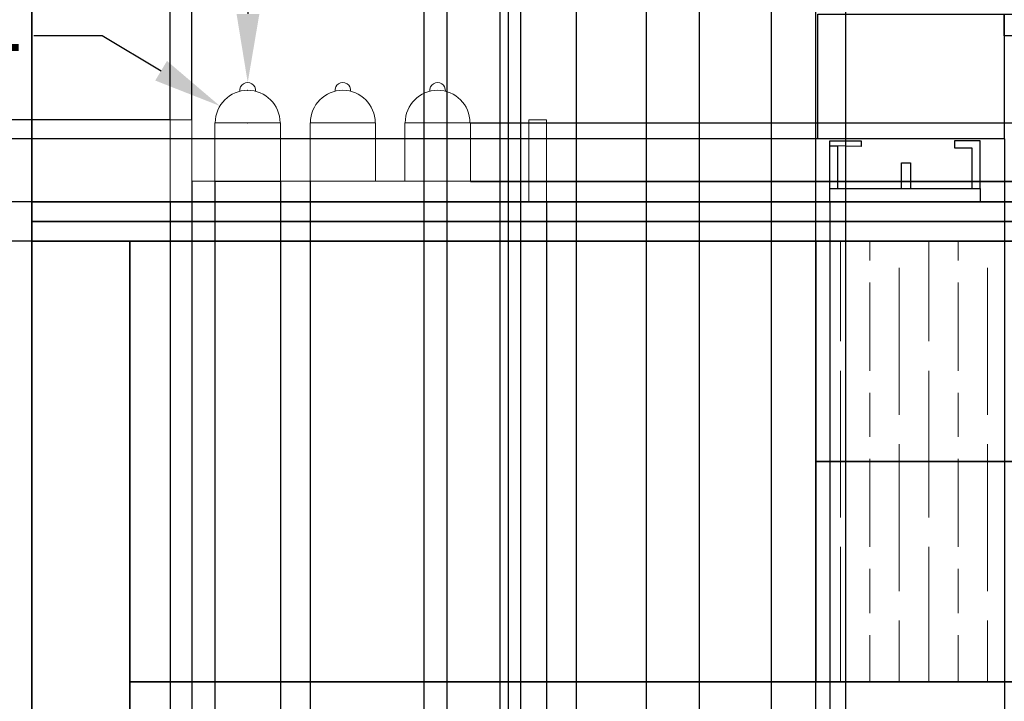
# Model space of a CAD drawing. Units: inches. Extents: x 600 to 5582, y -464 to 3142.
# Tile 3 of 9: x 1772 to 2777, y 532 to 1229. Entities that reach past the tile are written whole.
import ezdxf

# ---------------------------------------------------------------- set-up
doc = ezdxf.new("R2010")
doc.units = ezdxf.units.IN
doc.header["$MEASUREMENT"] = 0
for name, color, linetype, lineweight in [('A-ANNO-DIMS', 2, 'Continuous', 18), ('A-ELEV', 7, 'Continuous', 35), ('A-ELEV-PATT', 252, 'Continuous', 13), ('A-EQPM', 4, 'Continuous', 25), ('A-FURN', 8, 'Continuous', 18)]:
    doc.layers.add(name, color=color, linetype=linetype, lineweight=lineweight)
doc.styles.get("Standard").update_dxf_attribs({"font": 'arial.ttf'})
doc.dimstyles.get("Standard").update_dxf_attribs({"dimtxt": 70, "dimasz": 70, "dimexe": 0.18, "dimexo": 0.0625, "dimgap": 0.09, "dimtad": 0, "dimtih": 1, "dimtoh": 1, "dimdec": 0, "dimzin": 0, "dimdsep": 46, "dimtxsty": 'Standard', "dimcen": 0.09, "dimadec": 0, "dimazin": 0, "dimtfac": 1, "dimtdec": 0, "dimtofl": 0, "dimtmove": 0, "dimatfit": 3, "dimfxl": 1, "dimtolj": 1, "dimtzin": 0, "dimarcsym": 0})

# ---------------------------------------------------------------- blocks, each defined once
blk = doc.blocks.new('HOB-BURNER')
for p, q in [((0, 13.8), (0, 62.4)), ((0, 62.4), (31.8, 62.4)), ((31.8, 62.4), (31.8, 56.6)), ((153.5, 62.4), (127.3, 62.4)), ((127.3, 62.4), (127.3, 55.3)), ((153.5, 13.8), (153.5, 62.4)), ((31.8, 56.6), (0, 57.4)), ((0, 57.4), (7.8, 57.2)), ((7.8, 57.2), (7.8, 13.8)), ((127.3, 55.3), (144.9, 55.3)), ((144.9, 55.3), (144.9, 13.8)), ((73.1, 13.8), (73.1, 39.8)), ((73.1, 39.8), (82.4, 39.8)), ((82.4, 39.8), (82.4, 13.8)), ((7.8, 13.8), (73.1, 13.8)), ((82.4, 13.8), (153.5, 13.8))]:
    blk.add_line(p, q)
blk.add_lwpolyline([(0, 13.8), (153.5, 13.8), (153.5, 0), (0, 0)], close=True)
blk = doc.blocks.new('*D25')
at = {"layer": 'A-ANNO-DIMS', "color": 0, "lineweight": -2, "transparency": 16777216}
for p, q in [((2584.7, 1680.8), (2584.7, -233.3)), ((2615, 1655.8), (2615, -233.3)), ((2514.7, -233.1), (2444.7, -233.1)), ((2685, -233.1), (2755, -233.1))]:
    blk.add_line(p, q, dxfattribs=at)
at = {"layer": 'A-ANNO-DIMS', "color": 0, "transparency": 16777216}
for points in [[(2514.7, -221.4), (2514.7, -244.7), (2584.7, -233.1)], [(2685, -221.4), (2685, -244.7), (2615, -233.1)]]:
    blk.add_solid(points, dxfattribs=at)
at = {"layer": 'Defpoints', "color": 0, "transparency": 16777216}
for p in [(2584.7, 1680.8), (2615, 1655.8), (2615, -233.1)]:
    blk.add_point(p, dxfattribs=at)
at = {"layer": 'A-ANNO-DIMS', "color": 0, "transparency": 16777216, "insert": (2873.3, -233.1), "char_height": 70, "attachment_point": 5}
blk.add_mtext('\\A1;30.28', dxfattribs=at)
blk = doc.blocks.new('*D57')
at = {"layer": 'A-ANNO-DIMS', "color": 0, "lineweight": -2, "transparency": 16777216}
for p, q in [((5220.2, 622.4), (5220.2, 692.4)), ((5220.2, 692.4), (5290.2, 692.4)), ((1884.8, 552.4), (5220.4, 552.4)), ((1884.8, 512.4), (5220.4, 512.4)), ((5220.2, 442.4), (5220.2, 372.4))]:
    blk.add_line(p, q, dxfattribs=at)
at = {"layer": 'A-ANNO-DIMS', "color": 0, "transparency": 16777216}
for points in [[(5208.6, 622.4), (5231.9, 622.4), (5220.2, 552.4)], [(5208.6, 442.4), (5231.9, 442.4), (5220.2, 512.4)]]:
    blk.add_solid(points, dxfattribs=at)
at = {"layer": 'Defpoints', "color": 0, "transparency": 16777216}
for p in [(1884.7, 552.4), (5220.2, 552.4), (1884.7, 512.4)]:
    blk.add_point(p, dxfattribs=at)
at = {"layer": 'A-ANNO-DIMS', "color": 0, "transparency": 16777216, "insert": (5341.8, 692.4), "char_height": 70, "attachment_point": 5}
blk.add_mtext('\\A1;40', dxfattribs=at)
blk = doc.blocks.new('*D65')
at = {"layer": 'A-ANNO-DIMS', "color": 0, "lineweight": -2, "transparency": 16777216}
for p, q in [((1784.7, 2352.4), (1784.7, -233.3)), ((2184.7, 2352.4), (2184.7, -233.3)), ((1714.7, -233.1), (1644.7, -233.1)), ((2254.7, -233.1), (2324.7, -233.1))]:
    blk.add_line(p, q, dxfattribs=at)
at = {"layer": 'A-ANNO-DIMS', "color": 0, "transparency": 16777216}
for points in [[(1714.7, -221.4), (1714.7, -244.7), (1784.7, -233.1)], [(2254.7, -221.4), (2254.7, -244.7), (2184.7, -233.1)]]:
    blk.add_solid(points, dxfattribs=at)
at = {"layer": 'Defpoints', "color": 0, "transparency": 16777216}
for p in [(1784.7, 2352.4), (2184.7, 2352.4), (2184.7, -233.1)]:
    blk.add_point(p, dxfattribs=at)
at = {"layer": 'A-ANNO-DIMS', "color": 0, "transparency": 16777216, "insert": (1984.7, -233.1), "char_height": 70, "attachment_point": 5}
blk.add_mtext('\\A1;400.00', dxfattribs=at)
blk = doc.blocks.new('*D68')
at = {"layer": 'A-ANNO-DIMS', "color": 0, "lineweight": -2, "transparency": 16777216}
for p, q in [((2777.3, 1106.8), (2777.3, -233.3)), ((2584.7, 1002.4), (2584.7, -233.3)), ((2654.7, -233.1), (2707.3, -233.1)), ((2777.3, -233.1), (2847.3, -233.1))]:
    blk.add_line(p, q, dxfattribs=at)
at = {"layer": 'A-ANNO-DIMS', "color": 0, "transparency": 16777216}
for points in [[(2654.7, -221.4), (2654.7, -244.7), (2584.7, -233.1)], [(2707.3, -221.4), (2707.3, -244.7), (2777.3, -233.1)]]:
    blk.add_solid(points, dxfattribs=at)
at = {"layer": 'Defpoints', "color": 0, "transparency": 16777216}
for p in [(2777.3, 1106.8), (2584.7, 1002.4), (2777.3, -233.1)]:
    blk.add_point(p, dxfattribs=at)
at = {"layer": 'A-ANNO-DIMS', "color": 0, "transparency": 16777216, "insert": (2982.6, -233.1), "char_height": 70, "attachment_point": 5}
blk.add_mtext('\\A1;192.51', dxfattribs=at)
blk = doc.blocks.new('*D70')
at = {"layer": 'A-ANNO-DIMS', "color": 0, "lineweight": -2, "transparency": 16777216}
for p, q in [((1149.2, 1176.8), (1149.2, 1246.8)), ((1149.2, 1246.8), (1219.2, 1246.8)), ((2586.9, 1106.8), (1149.1, 1106.8)), ((2599.2, 1042.4), (1149.1, 1042.4)), ((1149.2, 972.4), (1149.2, 902.4))]:
    blk.add_line(p, q, dxfattribs=at)
at = {"layer": 'A-ANNO-DIMS', "color": 0, "transparency": 16777216}
for points in [[(1137.6, 1176.8), (1160.9, 1176.8), (1149.2, 1106.8)], [(1137.6, 972.4), (1160.9, 972.4), (1149.2, 1042.4)]]:
    blk.add_solid(points, dxfattribs=at)
at = {"layer": 'Defpoints', "color": 0, "transparency": 16777216}
for p in [(1149.2, 1106.8), (2586.9, 1106.8), (2599.2, 1042.4)]:
    blk.add_point(p, dxfattribs=at)
at = {"layer": 'A-ANNO-DIMS', "color": 0, "transparency": 16777216, "insert": (1337.3, 1246.8), "char_height": 70, "attachment_point": 5}
blk.add_mtext('\\A1;64.42', dxfattribs=at)
blk = doc.blocks.new('*D73')
at = {"layer": 'A-ANNO-DIMS', "color": 0, "lineweight": -2, "transparency": 16777216}
for p, q in [((2599.2, 1042.4), (2599.2, -233.3)), ((2584.7, 1002.4), (2584.7, -233.3)), ((2514.7, -233.1), (2444.7, -233.1)), ((2669.2, -233.1), (2739.2, -233.1))]:
    blk.add_line(p, q, dxfattribs=at)
at = {"layer": 'A-ANNO-DIMS', "color": 0, "transparency": 16777216}
for points in [[(2514.7, -221.4), (2514.7, -244.7), (2584.7, -233.1)], [(2669.2, -221.4), (2669.2, -244.7), (2599.2, -233.1)]]:
    blk.add_solid(points, dxfattribs=at)
at = {"layer": 'Defpoints', "color": 0, "transparency": 16777216}
for p in [(2599.2, 1042.4), (2584.7, 1002.4), (2599.2, -233.1)]:
    blk.add_point(p, dxfattribs=at)
at = {"layer": 'A-ANNO-DIMS', "color": 0, "transparency": 16777216, "insert": (2854, -233.1), "char_height": 70, "attachment_point": 5}
blk.add_mtext('\\A1;14.50', dxfattribs=at)
blk = doc.blocks.new('*D74')
at = {"layer": 'A-ANNO-DIMS', "color": 0, "lineweight": -2, "transparency": 16777216}
for p, q in [((2599.2, 1042.4), (2599.2, -233.3)), ((2884.4, 1042.4), (2884.4, -233.3)), ((2669.2, -233.1), (2814.4, -233.1)), ((2884.4, -233.1), (2954.4, -233.1))]:
    blk.add_line(p, q, dxfattribs=at)
at = {"layer": 'A-ANNO-DIMS', "color": 0, "transparency": 16777216}
for points in [[(2669.2, -221.4), (2669.2, -244.7), (2599.2, -233.1)], [(2814.4, -221.4), (2814.4, -244.7), (2884.4, -233.1)]]:
    blk.add_solid(points, dxfattribs=at)
at = {"layer": 'Defpoints', "color": 0, "transparency": 16777216}
for p in [(2599.2, 1042.4), (2884.4, 1042.4), (2884.4, -233.1)]:
    blk.add_point(p, dxfattribs=at)
at = {"layer": 'A-ANNO-DIMS', "color": 0, "transparency": 16777216, "insert": (3100, -233.1), "char_height": 70, "attachment_point": 5}
blk.add_mtext('\\A1;285.12', dxfattribs=at)
blk = doc.blocks.new('*D75')
at = {"layer": 'A-ANNO-DIMS', "color": 0, "lineweight": -2, "transparency": 16777216}
for p, q in [((2884.4, 1042.4), (2884.4, -233.3)), ((3196.2, 1042.4), (3196.2, -233.3)), ((2814.4, -233.1), (2744.4, -233.1)), ((3266.2, -233.1), (3336.2, -233.1))]:
    blk.add_line(p, q, dxfattribs=at)
at = {"layer": 'A-ANNO-DIMS', "color": 0, "transparency": 16777216}
for points in [[(2814.4, -221.4), (2814.4, -244.7), (2884.4, -233.1)], [(3266.2, -221.4), (3266.2, -244.7), (3196.2, -233.1)]]:
    blk.add_solid(points, dxfattribs=at)
at = {"layer": 'Defpoints', "color": 0, "transparency": 16777216}
for p in [(2884.4, 1042.4), (3196.2, 1042.4), (3196.2, -233.1)]:
    blk.add_point(p, dxfattribs=at)
at = {"layer": 'A-ANNO-DIMS', "color": 0, "transparency": 16777216, "insert": (3040.3, -233.1), "char_height": 70, "attachment_point": 5}
blk.add_mtext('\\A1;311.87', dxfattribs=at)
blk = doc.blocks.new('*D76')
at = {"layer": 'A-ANNO-DIMS', "color": 0, "lineweight": -2, "transparency": 16777216}
for p, q in [((1149.2, 1112.4), (1149.2, 1182.4)), ((1149.2, 1182.4), (1219.2, 1182.4)), ((1784.7, 1042.4), (1149.1, 1042.4)), ((1784.7, 1002.4), (1149.1, 1002.4)), ((1149.2, 932.4), (1149.2, 862.4))]:
    blk.add_line(p, q, dxfattribs=at)
at = {"layer": 'A-ANNO-DIMS', "color": 0, "transparency": 16777216}
for points in [[(1137.6, 1112.4), (1160.9, 1112.4), (1149.2, 1042.4)], [(1137.6, 932.4), (1160.9, 932.4), (1149.2, 1002.4)]]:
    blk.add_solid(points, dxfattribs=at)
at = {"layer": 'Defpoints', "color": 0, "transparency": 16777216}
for p in [(1149.2, 1042.4), (1784.7, 1042.4), (1784.7, 1002.4)]:
    blk.add_point(p, dxfattribs=at)
at = {"layer": 'A-ANNO-DIMS', "color": 0, "transparency": 16777216, "insert": (1338.7, 1182.4), "char_height": 70, "attachment_point": 5}
blk.add_mtext('\\A1;40.00', dxfattribs=at)
blk = doc.blocks.new('*D77')
at = {"layer": 'A-ANNO-DIMS', "color": 0, "lineweight": -2, "transparency": 16777216}
for p, q in [((1784.7, 1042.4), (1784.7, -233.3)), ((1925.7, 1042.4), (1925.7, -233.3)), ((1854.7, -233.1), (1855.7, -233.1)), ((1925.7, -233.1), (1995.7, -233.1))]:
    blk.add_line(p, q, dxfattribs=at)
at = {"layer": 'A-ANNO-DIMS', "color": 0, "transparency": 16777216}
for points in [[(1854.7, -221.4), (1854.7, -244.7), (1784.7, -233.1)], [(1855.7, -221.4), (1855.7, -244.7), (1925.7, -233.1)]]:
    blk.add_solid(points, dxfattribs=at)
at = {"layer": 'Defpoints', "color": 0, "transparency": 16777216}
for p in [(1784.7, 1042.4), (1925.7, 1042.4), (1925.7, -233.1)]:
    blk.add_point(p, dxfattribs=at)
at = {"layer": 'A-ANNO-DIMS', "color": 0, "transparency": 16777216, "insert": (2138.1, -233.1), "char_height": 70, "attachment_point": 5}
blk.add_mtext('\\A1;140.95', dxfattribs=at)
blk = doc.blocks.new('*D78')
at = {"layer": 'A-ANNO-DIMS', "color": 0, "lineweight": -2, "transparency": 16777216}
for p, q in [((1925.7, 1042.4), (1925.7, -233.3)), ((2310, 1042.4), (2310, -233.3)), ((1855.7, -233.1), (1785.7, -233.1)), ((2380, -233.1), (2450, -233.1))]:
    blk.add_line(p, q, dxfattribs=at)
at = {"layer": 'A-ANNO-DIMS', "color": 0, "transparency": 16777216}
for points in [[(1855.7, -221.4), (1855.7, -244.7), (1925.7, -233.1)], [(2380, -221.4), (2380, -244.7), (2310, -233.1)]]:
    blk.add_solid(points, dxfattribs=at)
at = {"layer": 'Defpoints', "color": 0, "transparency": 16777216}
for p in [(1925.7, 1042.4), (2310, 1042.4), (2310, -233.1)]:
    blk.add_point(p, dxfattribs=at)
at = {"layer": 'A-ANNO-DIMS', "color": 0, "transparency": 16777216, "insert": (2117.9, -233.1), "char_height": 70, "attachment_point": 5}
blk.add_mtext('\\A1;384.34', dxfattribs=at)
blk = doc.blocks.new('*D79')
at = {"layer": 'A-ANNO-DIMS', "color": 0, "lineweight": -2, "transparency": 16777216}
for p, q in [((1855.7, 2987.9), (1785.7, 2987.9)), ((1925.7, 1126.2), (1925.7, 2988.1)), ((1947.9, 1126.2), (1947.9, 2988.1)), ((2017.9, 2987.9), (2087.9, 2987.9))]:
    blk.add_line(p, q, dxfattribs=at)
at = {"layer": 'A-ANNO-DIMS', "color": 0, "transparency": 16777216}
for points in [[(1855.7, 2999.6), (1855.7, 2976.3), (1925.7, 2987.9)], [(2017.9, 2999.6), (2017.9, 2976.3), (1947.9, 2987.9)]]:
    blk.add_solid(points, dxfattribs=at)
at = {"layer": 'Defpoints', "color": 0, "transparency": 16777216}
for p in [(1947.9, 2987.9), (1925.7, 1126.1), (1947.9, 1126.1)]:
    blk.add_point(p, dxfattribs=at)
at = {"layer": 'A-ANNO-DIMS', "color": 0, "transparency": 16777216, "insert": (2234.2, 2987.9), "char_height": 70, "attachment_point": 5}
blk.add_mtext('\\A1;22.235', dxfattribs=at)
blk = doc.blocks.new('*D80')
at = {"layer": 'A-ANNO-DIMS', "color": 0, "lineweight": -2, "transparency": 16777216}
for p, q in [((1149.2, 1196.1), (1149.2, 1266.1)), ((1925.6, 1126.1), (1149.1, 1126.1)), ((1925.6, 1042.4), (1149.1, 1042.4)), ((1149.2, 972.4), (1149.2, 902.4))]:
    blk.add_line(p, q, dxfattribs=at)
at = {"layer": 'A-ANNO-DIMS', "color": 0, "transparency": 16777216}
for points in [[(1137.6, 1196.1), (1160.9, 1196.1), (1149.2, 1126.1)], [(1137.6, 972.4), (1160.9, 972.4), (1149.2, 1042.4)]]:
    blk.add_solid(points, dxfattribs=at)
at = {"layer": 'Defpoints', "color": 0, "transparency": 16777216}
for p in [(1149.2, 1126.1), (1925.7, 1126.1), (1925.7, 1042.4)]:
    blk.add_point(p, dxfattribs=at)
at = {"layer": 'A-ANNO-DIMS', "color": 0, "transparency": 16777216, "insert": (1149.2, 1084.3), "char_height": 70, "attachment_point": 5}
blk.add_mtext('\\A1;83.69', dxfattribs=at)
blk = doc.blocks.new('*D81')
at = {"layer": 'A-ANNO-DIMS', "color": 0, "lineweight": -2, "transparency": 16777216}
for p, q in [((5220.2, 1133.7), (5220.2, 1203.7)), ((5220.2, 1203.7), (5290.2, 1203.7)), ((2292.1, 1063.7), (5220.4, 1063.7)), ((2310.1, 1042.4), (5220.4, 1042.4)), ((5220.2, 972.4), (5220.2, 902.4))]:
    blk.add_line(p, q, dxfattribs=at)
at = {"layer": 'A-ANNO-DIMS', "color": 0, "transparency": 16777216}
for points in [[(5208.6, 1133.7), (5231.9, 1133.7), (5220.2, 1063.7)], [(5208.6, 972.4), (5231.9, 972.4), (5220.2, 1042.4)]]:
    blk.add_solid(points, dxfattribs=at)
at = {"layer": 'Defpoints', "color": 0, "transparency": 16777216}
for p in [(2292, 1063.7), (5220.2, 1063.7), (2310, 1042.4)]:
    blk.add_point(p, dxfattribs=at)
at = {"layer": 'A-ANNO-DIMS', "color": 0, "transparency": 16777216, "insert": (5409, 1203.7), "char_height": 70, "attachment_point": 5}
blk.add_mtext('\\A1;21.26', dxfattribs=at)
blk = doc.blocks.new('*D82')
at = {"layer": 'A-ANNO-DIMS', "color": 0, "lineweight": -2, "transparency": 16777216}
for p, q in [((1947.9, 1063.6), (1947.9, -233.3)), ((1971.5, 1063.3), (1971.5, -233.3)), ((1877.9, -233.1), (1807.9, -233.1)), ((2041.5, -233.1), (2111.5, -233.1))]:
    blk.add_line(p, q, dxfattribs=at)
at = {"layer": 'A-ANNO-DIMS', "color": 0, "transparency": 16777216}
for points in [[(1877.9, -221.4), (1877.9, -244.7), (1947.9, -233.1)], [(2041.5, -221.4), (2041.5, -244.7), (1971.5, -233.1)]]:
    blk.add_solid(points, dxfattribs=at)
at = {"layer": 'Defpoints', "color": 0, "transparency": 16777216}
for p in [(1947.9, 1063.7), (1971.5, 1063.4), (1971.5, -233.1)]:
    blk.add_point(p, dxfattribs=at)
at = {"layer": 'A-ANNO-DIMS', "color": 0, "transparency": 16777216, "insert": (2230.4, -233.1), "char_height": 70, "attachment_point": 5}
blk.add_mtext('\\A1;23.59', dxfattribs=at)
blk = doc.blocks.new('*D83')
at = {"layer": 'A-ANNO-DIMS', "color": 0, "lineweight": -2, "transparency": 16777216}
for p, q in [((1971.5, 1063.3), (1971.5, -233.3)), ((2038.4, 1063.3), (2038.4, -233.3)), ((1901.5, -233.1), (1831.5, -233.1)), ((2108.4, -233.1), (2178.4, -233.1))]:
    blk.add_line(p, q, dxfattribs=at)
at = {"layer": 'A-ANNO-DIMS', "color": 0, "transparency": 16777216}
for points in [[(1901.5, -221.4), (1901.5, -244.7), (1971.5, -233.1)], [(2108.4, -221.4), (2108.4, -244.7), (2038.4, -233.1)]]:
    blk.add_solid(points, dxfattribs=at)
at = {"layer": 'Defpoints', "color": 0, "transparency": 16777216}
for p in [(1971.5, 1063.4), (2038.4, 1063.4), (2038.4, -233.1)]:
    blk.add_point(p, dxfattribs=at)
at = {"layer": 'A-ANNO-DIMS', "color": 0, "transparency": 16777216, "insert": (2296.9, -233.1), "char_height": 70, "attachment_point": 5}
blk.add_mtext('\\A1;66.88', dxfattribs=at)
blk = doc.blocks.new('*D84')
at = {"layer": 'A-ANNO-DIMS', "color": 0, "lineweight": -2, "transparency": 16777216}
for p, q in [((2038.4, 1063.3), (2038.4, -233.3)), ((2068.6, 1063.3), (2068.6, -233.3)), ((1968.4, -233.1), (1898.4, -233.1)), ((2138.6, -233.1), (2208.6, -233.1))]:
    blk.add_line(p, q, dxfattribs=at)
at = {"layer": 'A-ANNO-DIMS', "color": 0, "transparency": 16777216}
for points in [[(1968.4, -221.4), (1968.4, -244.7), (2038.4, -233.1)], [(2138.6, -221.4), (2138.6, -244.7), (2068.6, -233.1)]]:
    blk.add_solid(points, dxfattribs=at)
at = {"layer": 'Defpoints', "color": 0, "transparency": 16777216}
for p in [(2038.4, 1063.4), (2068.6, 1063.4), (2068.6, -233.1)]:
    blk.add_point(p, dxfattribs=at)
at = {"layer": 'A-ANNO-DIMS', "color": 0, "transparency": 16777216, "insert": (2354, -233.1), "char_height": 70, "attachment_point": 5}
blk.add_mtext('\\A1;30.213', dxfattribs=at)
blk = doc.blocks.new('*D85')
at = {"layer": 'A-ANNO-DIMS', "color": 0, "lineweight": -2, "transparency": 16777216}
for p, q in [((5220.2, 1193.3), (5220.2, 1263.3)), ((5220.2, 1263.3), (5290.2, 1263.3)), ((2231.9, 1123.3), (5220.4, 1123.3)), ((2232.3, 1063.4), (5220.4, 1063.4)), ((5220.2, 993.4), (5220.2, 923.4))]:
    blk.add_line(p, q, dxfattribs=at)
at = {"layer": 'A-ANNO-DIMS', "color": 0, "transparency": 16777216}
for points in [[(5208.6, 1193.3), (5231.9, 1193.3), (5220.2, 1123.3)], [(5208.6, 993.4), (5231.9, 993.4), (5220.2, 1063.4)]]:
    blk.add_solid(points, dxfattribs=at)
at = {"layer": 'Defpoints', "color": 0, "transparency": 16777216}
for p in [(2231.8, 1123.3), (5220.2, 1123.3), (2232.2, 1063.4)]:
    blk.add_point(p, dxfattribs=at)
at = {"layer": 'A-ANNO-DIMS', "color": 0, "transparency": 16777216, "insert": (5408.5, 1263.3), "char_height": 70, "attachment_point": 5}
blk.add_mtext('\\A1;59.99', dxfattribs=at)
blk = doc.blocks.new('*D92')
at = {"layer": 'A-ANNO-DIMS', "color": 0, "lineweight": -2, "transparency": 16777216}
for p, q in [((2208.2, 1533.4), (2208.2, -233.3)), ((2271, 1533.4), (2271, -233.3)), ((2138.2, -233.1), (2068.2, -233.1)), ((2341, -233.1), (2411, -233.1))]:
    blk.add_line(p, q, dxfattribs=at)
at = {"layer": 'A-ANNO-DIMS', "color": 0, "transparency": 16777216}
for points in [[(2138.2, -221.4), (2138.2, -244.7), (2208.2, -233.1)], [(2341, -221.4), (2341, -244.7), (2271, -233.1)]]:
    blk.add_solid(points, dxfattribs=at)
at = {"layer": 'Defpoints', "color": 0, "transparency": 16777216}
for p in [(2208.2, 1533.5), (2271, 1533.5), (2271, -233.1)]:
    blk.add_point(p, dxfattribs=at)
at = {"layer": 'A-ANNO-DIMS', "color": 0, "transparency": 16777216, "insert": (2529.3, -233.1), "char_height": 70, "attachment_point": 5}
blk.add_mtext('\\A1;62.77', dxfattribs=at)
blk = doc.blocks.new('*D93')
at = {"layer": 'A-ANNO-DIMS', "color": 0, "lineweight": -2, "transparency": 16777216}
for p, q in [((2271, 1533.4), (2271, -233.3)), ((2340.4, 1533.4), (2340.4, -233.3)), ((2201, -233.1), (2131, -233.1)), ((2410.4, -233.1), (2480.4, -233.1))]:
    blk.add_line(p, q, dxfattribs=at)
at = {"layer": 'A-ANNO-DIMS', "color": 0, "transparency": 16777216}
for points in [[(2201, -221.4), (2201, -244.7), (2271, -233.1)], [(2410.4, -221.4), (2410.4, -244.7), (2340.4, -233.1)]]:
    blk.add_solid(points, dxfattribs=at)
at = {"layer": 'Defpoints', "color": 0, "transparency": 16777216}
for p in [(2271, 1533.5), (2340.4, 1533.5), (2340.4, -233.1)]:
    blk.add_point(p, dxfattribs=at)
at = {"layer": 'A-ANNO-DIMS', "color": 0, "transparency": 16777216, "insert": (2598.6, -233.1), "char_height": 70, "attachment_point": 5}
blk.add_mtext('\\A1;69.40', dxfattribs=at)
blk = doc.blocks.new('*D94')
at = {"layer": 'A-ANNO-DIMS', "color": 0, "lineweight": -2, "transparency": 16777216}
for p, q in [((2340.4, 1533.4), (2340.4, -233.3)), ((2411.7, 1533.4), (2411.7, -233.3)), ((2270.4, -233.1), (2200.4, -233.1)), ((2481.7, -233.1), (2551.7, -233.1))]:
    blk.add_line(p, q, dxfattribs=at)
at = {"layer": 'A-ANNO-DIMS', "color": 0, "transparency": 16777216}
for points in [[(2270.4, -221.4), (2270.4, -244.7), (2340.4, -233.1)], [(2481.7, -221.4), (2481.7, -244.7), (2411.7, -233.1)]]:
    blk.add_solid(points, dxfattribs=at)
at = {"layer": 'Defpoints', "color": 0, "transparency": 16777216}
for p in [(2340.4, 1533.5), (2411.7, 1533.5), (2411.7, -233.1)]:
    blk.add_point(p, dxfattribs=at)
at = {"layer": 'A-ANNO-DIMS', "color": 0, "transparency": 16777216, "insert": (2669.5, -233.1), "char_height": 70, "attachment_point": 5}
blk.add_mtext('\\A1;71.34', dxfattribs=at)
blk = doc.blocks.new('*D95')
at = {"layer": 'A-ANNO-DIMS', "color": 0, "lineweight": -2, "transparency": 16777216}
for p, q in [((2411.7, 1533.4), (2411.7, -233.3)), ((2465.8, 1533.4), (2465.8, -233.3)), ((2341.7, -233.1), (2271.7, -233.1)), ((2535.8, -233.1), (2605.8, -233.1))]:
    blk.add_line(p, q, dxfattribs=at)
at = {"layer": 'A-ANNO-DIMS', "color": 0, "transparency": 16777216}
for points in [[(2341.7, -221.4), (2341.7, -244.7), (2411.7, -233.1)], [(2535.8, -221.4), (2535.8, -244.7), (2465.8, -233.1)]]:
    blk.add_solid(points, dxfattribs=at)
at = {"layer": 'Defpoints', "color": 0, "transparency": 16777216}
for p in [(2411.7, 1533.5), (2465.8, 1533.5), (2465.8, -233.1)]:
    blk.add_point(p, dxfattribs=at)
at = {"layer": 'A-ANNO-DIMS', "color": 0, "transparency": 16777216, "insert": (2724, -233.1), "char_height": 70, "attachment_point": 5}
blk.add_mtext('\\A1;54.13', dxfattribs=at)
blk = doc.blocks.new('*D96')
at = {"layer": 'A-ANNO-DIMS', "color": 0, "lineweight": -2, "transparency": 16777216}
for p, q in [((2465.8, 1533.4), (2465.8, -233.3)), ((2539.2, 1533.4), (2539.2, -233.3)), ((2395.8, -233.1), (2325.8, -233.1)), ((2609.2, -233.1), (2679.2, -233.1))]:
    blk.add_line(p, q, dxfattribs=at)
at = {"layer": 'A-ANNO-DIMS', "color": 0, "transparency": 16777216}
for points in [[(2395.8, -221.4), (2395.8, -244.7), (2465.8, -233.1)], [(2609.2, -221.4), (2609.2, -244.7), (2539.2, -233.1)]]:
    blk.add_solid(points, dxfattribs=at)
at = {"layer": 'Defpoints', "color": 0, "transparency": 16777216}
for p in [(2465.8, 1533.5), (2539.2, 1533.5), (2539.2, -233.1)]:
    blk.add_point(p, dxfattribs=at)
at = {"layer": 'A-ANNO-DIMS', "color": 0, "transparency": 16777216, "insert": (2797.1, -233.1), "char_height": 70, "attachment_point": 5}
blk.add_mtext('\\A1;73.33', dxfattribs=at)
blk = doc.blocks.new('*D100')
at = {"layer": 'A-ANNO-DIMS', "color": 0, "lineweight": -2, "transparency": 16777216}
for p, q in [((2262.3, 1439.7), (2262.3, -233.3)), ((2283.5, 1439.7), (2283.5, -233.3)), ((2192.3, -233.1), (2122.3, -233.1)), ((2353.5, -233.1), (2423.5, -233.1))]:
    blk.add_line(p, q, dxfattribs=at)
at = {"layer": 'A-ANNO-DIMS', "color": 0, "transparency": 16777216}
for points in [[(2192.3, -221.4), (2192.3, -244.7), (2262.3, -233.1)], [(2353.5, -221.4), (2353.5, -244.7), (2283.5, -233.1)]]:
    blk.add_solid(points, dxfattribs=at)
at = {"layer": 'Defpoints', "color": 0, "transparency": 16777216}
for p in [(2262.3, 1439.7), (2283.5, 1439.7), (2283.5, -233.1)]:
    blk.add_point(p, dxfattribs=at)
at = {"layer": 'A-ANNO-DIMS', "color": 0, "transparency": 16777216, "insert": (2569.4, -233.1), "char_height": 70, "attachment_point": 5}
blk.add_mtext('\\A1;21.136', dxfattribs=at)
blk = doc.blocks.new('*D104')
at = {"layer": 'A-ANNO-DIMS', "color": 0, "lineweight": -2, "transparency": 16777216}
for p, q in [((1786.6, 1212.4), (1856.6, 1212.4)), ((1856.6, 1212.4), (1916.6, 1176.4)), ((2004.9, 1123.3), (2005.1, 1123.3)), ((2005, 1123.3), (2005, 1123.4))]:
    blk.add_line(p, q, dxfattribs=at)
at = {"layer": 'A-ANNO-DIMS', "color": 0, "transparency": 16777216}
blk.add_solid([(1922.6, 1186.4), (1910.6, 1166.4), (1976.6, 1140.4)], dxfattribs=at)
at = {"layer": 'Defpoints', "color": 0, "transparency": 16777216}
for p in [(1976.6, 1140.4), (2005, 1123.3)]:
    blk.add_point(p, dxfattribs=at)
at = {"layer": 'A-ANNO-DIMS', "color": 0, "transparency": 16777216, "insert": (1559.9, 1212.4), "char_height": 70, "attachment_point": 5}
blk.add_mtext('\\A1;3X R33.04', dxfattribs=at)
blk = doc.blocks.new('*D105')
at = {"layer": 'A-ANNO-DIMS', "color": 0, "lineweight": -2, "transparency": 16777216}
for p, q in [((2005.5, 1304.4), (2005.2, 1234.4)), ((2075.5, 1304.4), (2005.5, 1304.4)), ((2004.9, 1156.4), (2005.1, 1156.4)), ((2005, 1156.3), (2005, 1156.5))]:
    blk.add_line(p, q, dxfattribs=at)
at = {"layer": 'A-ANNO-DIMS', "color": 0, "transparency": 16777216}
blk.add_solid([(1993.6, 1234.4), (2016.9, 1234.4), (2005, 1164.4)], dxfattribs=at)
at = {"layer": 'Defpoints', "color": 0, "transparency": 16777216}
for p in [(2005, 1164.4), (2005, 1156.4)]:
    blk.add_point(p, dxfattribs=at)
at = {"layer": 'A-ANNO-DIMS', "color": 0, "transparency": 16777216, "insert": (2302.6, 1304.4), "char_height": 70, "attachment_point": 5}
blk.add_mtext('\\A1;3X R8.005', dxfattribs=at)

msp = doc.modelspace()

# ---------------------------------------------------------------- hatches: boundary and pattern name
at = {"layer": 'A-ELEV-PATT'}
h = msp.add_hatch(dxfattribs=at)
h.set_pattern_fill('GOST_WOOD', color=256, scale=15)
h.set_pattern_definition([(90, (0, 0), (90, -6e-15), [150, -30]), (90, (30, -30), (90, -6e-15), [90, -22.5, 45, -22.5]), (90, (60, -75), (90, -6e-15), [150, -30])])
h.paths.add_polyline_path([(4959.7485, 2752.4212), (1409.7485, 2752.4212), (1409.7485, 2352.4212), (1784.7485, 2352.4212), (4959.7485, 2352.4212)])
h.paths.add_polyline_path([(3384.7485, 1002.4212), (2584.7485, 1002.4212), (2584.7485, 777.4212), (3384.7485, 777.4212)])
h.paths.add_polyline_path([(3384.7485, 777.4212), (2584.7485, 777.4212), (2584.7485, 552.4212), (3384.7485, 552.4212)])
h.paths.add_polyline_path([(3384.7485, 512.4212), (2584.7485, 512.4212), (2584.7485, 102.4212), (3384.7485, 102.4212)])
h = msp.add_hatch(dxfattribs=at)
h.set_pattern_fill('CROSS', color=256, scale=100)
h.paths.add_polyline_path([(1759.7485, 2327.4212), (1409.7485, 2327.4212), (1409.7485, 1967.4212), (1759.7485, 1967.4212)])
h.paths.add_polyline_path([(1759.7485, 1952.4212), (1409.7485, 1952.4212), (1409.7485, 1567.4212), (1759.7485, 1567.4212)])
h.paths.add_polyline_path([(1759.7485, 1552.4212), (1409.7485, 1552.4212), (1409.7485, 1167.4212), (1759.7485, 1167.4212)])
h.paths.add_polyline_path([(1759.7485, 1152.4212), (1409.7485, 1152.4212), (1409.7485, 767.4212), (1759.7485, 767.4212)])
h.paths.add_polyline_path([(1759.7485, 752.4212), (1409.7485, 752.4212), (1409.7485, 367.4212), (1759.7485, 367.4212)])
h.paths.add_polyline_path([(1759.7485, 352.4212), (1409.7485, 352.4212), (1409.7485, 142.4212), (1759.7485, 142.4212)])
h.paths.add_polyline_path([(3759.7485, 1977.4212), (3409.7485, 1977.4212), (3409.7485, 1627.4212), (3759.7485, 1627.4212)])
h.paths.add_polyline_path([(3714.7508, 1954.858, -1), (3750.8891, 1954.858, -1)], flags=16)
h.paths.add_polyline_path([(3759.7485, 2327.4212), (3409.7485, 2327.4212), (3409.7485, 2002.4212), (3759.7485, 2002.4212)])
h.paths.add_polyline_path([(4159.7485, 2327.4212), (3809.7485, 2327.4212), (3809.7485, 2002.4212), (4159.7485, 2002.4212)])
h.paths.add_polyline_path([(4159.7485, 1977.4212), (3809.7485, 1977.4212), (3813.5467, 1954.858, -1), (3849.685, 1954.858, -1), (3813.5467, 1954.858), (3809.7485, 1627.4212), (4159.7485, 1627.4212)])
h.paths.add_polyline_path([(4559.7485, 2327.4212), (4184.7485, 2327.4212), (4184.7485, 2002.4212), (4559.7485, 2002.4212)])
h.paths.add_polyline_path([(4559.7485, 1977.4212), (4184.7485, 1977.4212), (4184.7485, 1627.4212), (4559.7485, 1627.4212)])
h.paths.add_polyline_path([(4517.0704, 1954.858, -1), (4553.2087, 1954.858, -1)], flags=16)
h.paths.add_polyline_path([(4959.7485, 2327.4212), (4609.7485, 2327.4212), (4609.7485, 2002.4212), (4959.7485, 2002.4212)])
h.paths.add_polyline_path([(4959.7485, 1977.4212), (4609.7485, 1977.4212), (4609.7485, 1627.4212), (4959.7485, 1627.4212)])
h.paths.add_polyline_path([(4619.5464, 1954.858, -1), (4655.6847, 1954.858, -1)], flags=16)

# ---------------------------------------------------------------- linework, layer by layer
at = {"layer": 'A-ELEV'}
for p, q in [((4984.7485, 1042.4212), (1784.7485, 1042.4212)), ((4984.7485, 1022.4212), (1784.7485, 1022.4212)), ((4984.7485, 1002.4212), (1784.7485, 1002.4212)), ((1884.7485, 102.4212), (1884.7485, 1002.4212)), ((2584.7485, 552.4212), (2584.7485, 1002.4212)), ((2584.7485, 777.4212), (3384.7485, 777.4212)), ((4184.7485, 552.4212), (1884.7485, 552.4212))]:
    msp.add_line(p, q, dxfattribs=at)
msp.add_lwpolyline([(1784.7485, 2.4212), (1784.7485, 2352.4212), (1384.7485, 2352.4212), (1409.7485, 2327.4212), (1759.7485, 2327.4212), (1409.7485, 2327.4212), (1409.7485, 127.4212)], dxfattribs=at)
at = {"layer": 'A-EQPM'}
for points in [[(2586.9456, 1106.8415), (2586.9456, 1234.0488), (2777.2556, 1234.0488), (2777.2556, 1106.8415)], [(2777.2556, 1234.0488), (2947.8448, 1234.0488), (2947.8448, 1211.9616), (2777.2556, 1211.9616)]]:
    msp.add_lwpolyline(points, close=True, dxfattribs=at)
at = {"layer": 'A-FURN'}
for points in [[(1925.6996, 1042.4212), (1925.6996, 1042.4212), (1925.6996, 1126.1128), (1947.9344, 1126.1128), (1947.9344, 1042.4212), (1947.9344, 1063.682), (2292.0448, 1063.682), (2292.0448, 1042.4212)], [(2135.5031, 1063.362), (2135.5031, 1123.3472), (2068.6213, 1123.3472), (2068.6213, 1063.362)], [(2232.228, 1063.362), (2232.228, 1123.3472), (2165.3462, 1123.3472), (2165.3462, 1063.362)]]:
    msp.add_lwpolyline(points, dxfattribs=at)
for points in [[(2292.0448, 1126.1128), (2310.0444, 1126.1128), (2310.0444, 1042.4212), (2292.0448, 1042.4212)], [(1971.5262, 1063.362), (2038.408, 1063.362), (2038.408, 1123.3472), (1971.5262, 1123.3472)]]:
    msp.add_lwpolyline(points, close=True, dxfattribs=at)
for centre, radius, start, end in [((2004.9671, 1123.3472), 33.0405, 0, 180), ((2004.9671, 1156.3876), 8.0046, 353.042512, 186.957488), ((2102.0622, 1123.3472), 33.0405, 0, 180), ((2102.0622, 1156.3876), 8.0046, 353.042512, 186.957488), ((2198.7871, 1123.3472), 33.0405, 0, 180), ((2198.7871, 1156.3876), 8.0046, 353.042512, 186.957488)]:
    msp.add_arc(centre, radius, start, end, dxfattribs=at)

# ---------------------------------------------------------------- block references
at = {"layer": 'A-EQPM'}
msp.add_blockref('HOB-BURNER', (2599.25, 1042.42), dxfattribs=at)

# ---------------------------------------------------------------- dimensions: what is measured, and where the dimension line sits
at = {"layer": 'A-ANNO-DIMS'}
for base, p1, p2, override, picture, middle in [((1947.9344, 2987.9212), (1925.6996, 1126.1128), (1947.9344, 1126.1128), {"dimdec": 3, "dimlfac": 1, "dimrnd": 0, "dimzin": 0, "dimdsep": 46, "dimlunit": 2}, '*D79', (2234.1841, 2987.9212)), ((2184.7485, -233.0788), (1784.7485, 2352.4212), (2184.7485, 2352.4212), {"dimdec": 2, "dimlfac": 1, "dimrnd": 0, "dimzin": 0, "dimdsep": 46, "dimlunit": 2}, '*D65', (1984.7485, -233.0788)), ((2615.026, -233.0788), (2584.7485, 1680.8271), (2615.026, 1655.8271), {"dimdec": 2, "dimlfac": 1, "dimrnd": 0, "dimzin": 0, "dimdsep": 46, "dimlunit": 2}, '*D25', (2873.2709, -233.0788)), ((2270.9593, -233.0788), (2208.185, 1533.4874), (2270.9593, 1533.4874), {"dimdec": 2, "dimlfac": 1, "dimrnd": 0, "dimzin": 0, "dimdsep": 46, "dimlunit": 2}, '*D92', (2529.3474, -233.0788)), ((2340.3598, -233.0788), (2270.9593, 1533.4874), (2340.3598, 1533.4874), {"dimdec": 2, "dimlfac": 1, "dimrnd": 0, "dimzin": 0, "dimdsep": 46, "dimlunit": 2}, '*D93', (2598.6285, -233.0788)), ((2411.7034, -233.0788), (2340.3598, 1533.4874), (2411.7034, 1533.4874), {"dimdec": 2, "dimlfac": 1, "dimrnd": 0, "dimzin": 0, "dimdsep": 46, "dimlunit": 2}, '*D94', (2669.4707, -233.0788)), ((2465.8357, -233.0788), (2411.7034, 1533.4874), (2465.8357, 1533.4874), {"dimdec": 2, "dimlfac": 1, "dimrnd": 0, "dimzin": 0, "dimdsep": 46, "dimlunit": 2}, '*D95', (2724.0328, -233.0788)), ((2539.1643, -233.0788), (2465.8357, 1533.4874), (2539.1643, 1533.4874), {"dimdec": 2, "dimlfac": 1, "dimrnd": 0, "dimzin": 0, "dimdsep": 46, "dimlunit": 2}, '*D96', (2797.0749, -233.0788)), ((2283.4705, -233.0788), (2262.3346, 1439.718), (2283.4705, 1439.718), {"dimdec": 3, "dimlfac": 1, "dimrnd": 0, "dimzin": 0, "dimdsep": 46, "dimlunit": 2}, '*D100', (2569.4336, -233.0788)), ((2777.2556, -233.0788), (2584.7485, 1002.4212), (2777.2556, 1106.8415), {"dimdec": 2, "dimlfac": 1, "dimrnd": 0, "dimzin": 0, "dimdsep": 46, "dimlunit": 2}, '*D68', (2982.5946, -233.0788)), ((1971.5262, -233.0788), (1947.9344, 1063.682), (1971.5262, 1063.362), {"dimdec": 2, "dimlfac": 1, "dimrnd": 0, "dimzin": 0, "dimdsep": 46, "dimlunit": 2}, '*D82', (2230.3918, -233.0788)), ((2038.408, -233.0788), (1971.5262, 1063.362), (2038.408, 1063.362), {"dimdec": 2, "dimlfac": 1, "dimrnd": 0, "dimzin": 0, "dimdsep": 46, "dimlunit": 2}, '*D83', (2296.8677, -233.0788)), ((2068.6213, -233.0788), (2038.408, 1063.362), (2068.6213, 1063.362), {"dimdec": 3, "dimlfac": 1, "dimrnd": 0, "dimzin": 0, "dimdsep": 46, "dimlunit": 2}, '*D84', (2353.9875, -233.0788)), ((1925.6996, -233.0788), (1784.7485, 1042.4212), (1925.6996, 1042.4212), {"dimdec": 2, "dimlfac": 1, "dimrnd": 0, "dimzin": 0, "dimdsep": 46, "dimlunit": 2}, '*D77', (2138.0577, -233.0788)), ((2310.0444, -233.0788), (1925.6996, 1042.4212), (2310.0444, 1042.4212), {"dimdec": 2, "dimlfac": 1, "dimrnd": 0, "dimzin": 0, "dimdsep": 46, "dimlunit": 2}, '*D78', (2117.872, -233.0788)), ((2599.2497, -233.0788), (2584.7485, 1002.4212), (2599.2497, 1042.42), {"dimdec": 2, "dimlfac": 1, "dimrnd": 0, "dimzin": 0, "dimdsep": 46, "dimlunit": 2}, '*D73', (2854.0327, -233.0788)), ((2884.371, -233.0788), (2599.2497, 1042.42), (2884.371, 1042.4212), {"dimdec": 2, "dimlfac": 1, "dimrnd": 0, "dimzin": 0, "dimdsep": 46, "dimlunit": 2}, '*D74', (3099.9999, -233.0788)), ((3196.2381, -233.0788), (2884.371, 1042.4212), (3196.2381, 1042.4212), {"dimdec": 2, "dimlfac": 1, "dimrnd": 0, "dimzin": 0, "dimdsep": 46, "dimlunit": 2}, '*D75', (3040.3046, -233.0788))]:
    dim = msp.add_linear_dim(base=base, p1=p1, p2=p2, dimstyle='Standard', override=override, dxfattribs=at)
    dim.commit()
    dim.dimension.update_dxf_attribs({"geometry": picture, "text_midpoint": middle})
for center, mpoint, override, picture, middle in [((2004.9671, 1156.3876), (2004.9945, 1164.3922), {"dimdec": 3, "dimlfac": 1, "dimrnd": 0, "dimzin": 0, "dimdsep": 46, "dimlunit": 2}, '*D105', (2302.6098, 1304.3914)), ((2004.9671, 1123.3472), (1976.6406, 1140.3555), {"dimdec": 2, "dimlfac": 1, "dimrnd": 0, "dimzin": 0, "dimdsep": 46, "dimlunit": 2}, '*D104', (1559.8844, 1212.4236))]:
    dim = msp.add_radius_dim(center=center, mpoint=mpoint, text='3X <>', dimstyle='Standard', override=override, dxfattribs=at)
    dim.commit()
    dim.dimension.update_dxf_attribs({"geometry": picture, "text_midpoint": middle})
for base, p1, p2, override, picture, middle in [((5220.2485, 1123.3472), (2232.228, 1063.362), (2231.8275, 1123.3472), {"dimdec": 2, "dimlfac": 1, "dimrnd": 0, "dimzin": 0, "dimdsep": 46, "dimlunit": 2}, '*D85', (5408.5172, 1263.3472)), ((1149.2485, 1106.8415), (2599.2497, 1042.42), (2586.9456, 1106.8415), {"dimdec": 2, "dimlfac": 1, "dimrnd": 0, "dimzin": 0, "dimdsep": 46, "dimlunit": 2}, '*D70', (1337.2784, 1246.8415)), ((1149.2485, 1126.1128), (1925.6996, 1042.4212), (1925.6996, 1126.1128), {"dimdec": 2, "dimlfac": 1, "dimrnd": 0, "dimzin": 0, "dimdsep": 46, "dimlunit": 2}, '*D80', (1149.2485, 1084.267)), ((5220.2485, 1063.682), (2310.0444, 1042.4212), (2292.0448, 1063.682), {"dimdec": 2, "dimlfac": 1, "dimrnd": 0, "dimzin": 0, "dimdsep": 46, "dimlunit": 2}, '*D81', (5409.0186, 1203.682)), ((1149.2485, 1042.4212), (1784.7485, 1002.4212), (1784.7485, 1042.4212), {"dimdec": 2, "dimlfac": 1, "dimrnd": 0, "dimzin": 0, "dimdsep": 46, "dimlunit": 2}, '*D76', (1338.7348, 1182.4212)), ((5220.2485, 552.4212), (1884.7485, 512.4212), (1884.7485, 552.4212), {"dimdec": 0, "dimlfac": 1, "dimrnd": 0, "dimzin": 0, "dimdsep": 46, "dimlunit": 2}, '*D57', (5341.7641, 692.4212))]:
    dim = msp.add_linear_dim(base=base, p1=p1, p2=p2, angle=90, dimstyle='Standard', override=override, dxfattribs=at)
    dim.commit()
    dim.dimension.update_dxf_attribs({"geometry": picture, "text_midpoint": middle})

doc.saveas('drawing.dxf')
